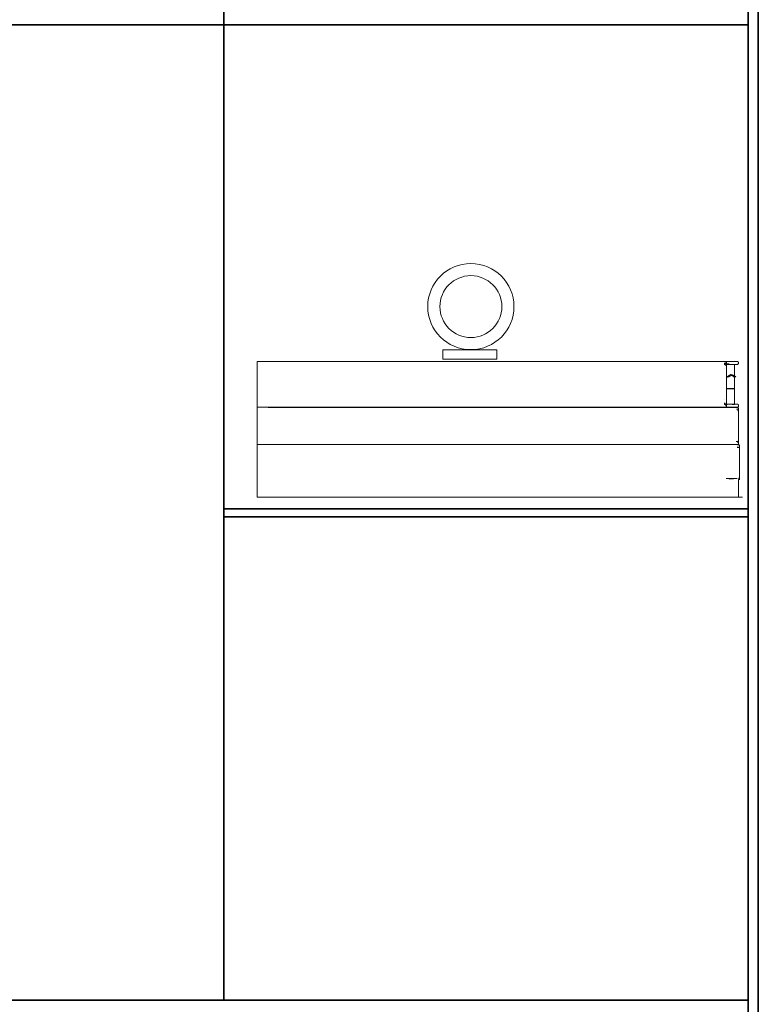
# Model space of a CAD drawing. Units: millimetres. Extents: x 2322 to 2394, y 1600 to 1790.
# Tile 3 of 5: x 2358 to 2394, y 1648 to 1696. Entities that reach past the tile are written whole.
import ezdxf

# ---------------------------------------------------------------- set-up
doc = ezdxf.new("R2010")
doc.units = ezdxf.units.MM
doc.layers.add('A-FURN', color=7, linetype='Continuous', lineweight=35)
doc.layers.add('A-FURN-ACCS', color=8, linetype='Continuous', lineweight=18)

msp = doc.modelspace()

# ---------------------------------------------------------------- linework, layer by layer
at = {"layer": 'A-FURN'}
for p, q in [((2393.58, 1755.925), (2393.58, 1599.925)), ((2393.08, 1755.425), (2393.08, 1600.425)), ((2367.535, 1701.437), (2367.535, 1648.381)), ((2322.08, 1695.937), (2393.08, 1695.937)), ((2393.08, 1695.937), (2393.08, 1600.425)), ((2393.08, 1695.937), (2393.08, 1648.381)), ((2367.535, 1672.346), (2393.08, 1672.346)), ((2367.535, 1671.946), (2393.08, 1671.946)), ((2393.08, 1648.381), (2322.08, 1648.381))]:
    msp.add_line(p, q, dxfattribs=at)
at = {"layer": 'A-FURN-ACCS'}
for p, q in [((2391.983, 1679.528), (2369.151, 1679.528)), ((2369.151, 1679.528), (2369.151, 1672.902)), ((2391.992, 1679.442), (2391.91, 1679.442)), ((2391.915, 1679.412), (2391.91, 1679.413)), ((2391.91, 1679.377), (2391.978, 1679.377)), ((2391.922, 1679.33), (2391.91, 1679.33)), ((2392.007, 1679.413), (2391.915, 1679.412)), ((2391.985, 1679.37), (2391.978, 1679.37)), ((2391.992, 1679.33), (2391.978, 1679.33)), ((2392.002, 1679.512), (2391.983, 1679.528)), ((2392.567, 1679.528), (2391.983, 1679.528)), ((2391.988, 1679.373), (2391.985, 1679.37)), ((2392.014, 1679.422), (2391.992, 1679.442)), ((2392.028, 1679.363), (2391.992, 1679.33)), ((2392.002, 1679.512), (2392.027, 1679.494)), ((2392.029, 1679.408), (2392.025, 1679.412)), ((2392.025, 1679.412), (2392.029, 1679.412)), ((2392.029, 1679.405), (2392.025, 1679.401)), ((2392.025, 1679.377), (2392.029, 1679.405)), ((2392.028, 1679.372), (2392.025, 1679.377)), ((2392.028, 1679.377), (2392.025, 1679.377)), ((2392.027, 1679.49), (2392.027, 1679.494)), ((2392.03, 1679.488), (2392.027, 1679.49)), ((2392.027, 1679.109), (2392.028, 1679.324)), ((2392.039, 1679.374), (2392.028, 1679.377)), ((2392.028, 1679.363), (2392.028, 1679.372)), ((2392.037, 1679.372), (2392.028, 1679.363)), ((2392.028, 1679.324), (2392.028, 1679.363)), ((2392.029, 1679.412), (2392.032, 1679.454)), ((2392.029, 1679.412), (2392.036, 1679.414)), ((2392.029, 1679.408), (2392.029, 1679.412)), ((2392.037, 1679.4), (2392.029, 1679.408)), ((2392.029, 1679.405), (2392.029, 1679.408)), ((2392.032, 1679.454), (2392.03, 1679.488)), ((2392.036, 1679.414), (2392.032, 1679.454)), ((2392.045, 1679.419), (2392.036, 1679.414)), ((2392.036, 1679.414), (2392.044, 1679.413)), ((2392.037, 1679.4), (2392.036, 1679.414)), ((2392.037, 1679.372), (2392.039, 1679.374)), ((2392.039, 1679.374), (2392.04, 1679.385)), ((2392.039, 1679.374), (2392.055, 1679.377)), ((2392.04, 1679.385), (2392.043, 1679.408)), ((2392.043, 1679.408), (2392.044, 1679.413)), ((2392.044, 1679.413), (2392.045, 1679.419)), ((2392.044, 1679.413), (2392.053, 1679.413)), ((2392.055, 1679.377), (2392.421, 1679.377)), ((2392.078, 1679.412), (2392.068, 1679.413)), ((2392.163, 1679.413), (2392.078, 1679.412)), ((2392.421, 1679.377), (2392.419, 1679.179)), ((2392.421, 1679.377), (2392.567, 1679.377)), ((2392.567, 1679.528), (2392.612, 1679.486)), ((2392.612, 1679.419), (2392.567, 1679.377)), ((2392.612, 1679.486), (2392.612, 1679.419)), ((2391.913, 1679.179), (2391.909, 1679.179)), ((2392.025, 1678.791), (2392.027, 1679.109)), ((2392.027, 1678.788), (2392.025, 1678.791)), ((2392.025, 1678.788), (2392.025, 1678.791)), ((2392.025, 1678.788), (2392.027, 1678.788)), ((2392.025, 1678.779), (2392.025, 1678.788)), ((2392.025, 1678.779), (2392.027, 1678.779)), ((2392.025, 1678.775), (2392.025, 1678.779)), ((2392.025, 1678.775), (2392.093, 1678.776)), ((2392.025, 1678.768), (2392.025, 1678.775)), ((2392.071, 1678.791), (2392.027, 1678.788)), ((2392.027, 1678.779), (2392.093, 1678.776)), ((2392.071, 1678.791), (2392.074, 1678.788)), ((2392.074, 1678.788), (2392.079, 1678.791)), ((2392.083, 1678.791), (2392.079, 1678.791)), ((2392.166, 1678.777), (2392.079, 1678.768)), ((2392.093, 1678.776), (2392.079, 1678.768)), ((2392.083, 1678.791), (2392.237, 1678.882)), ((2392.093, 1678.776), (2392.096, 1678.779)), ((2392.166, 1678.777), (2392.096, 1678.779)), ((2392.237, 1678.859), (2392.164, 1678.817)), ((2392.166, 1678.777), (2392.275, 1678.84)), ((2392.329, 1678.87), (2392.237, 1678.882)), ((2392.237, 1678.882), (2392.273, 1678.863)), ((2392.273, 1678.863), (2392.237, 1678.859)), ((2392.259, 1678.848), (2392.237, 1678.859)), ((2392.329, 1678.87), (2392.273, 1678.863)), ((2392.273, 1678.863), (2392.286, 1678.857)), ((2392.275, 1678.84), (2392.296, 1678.852)), ((2392.372, 1678.791), (2392.275, 1678.84)), ((2392.296, 1678.852), (2392.329, 1678.87)), ((2392.296, 1678.852), (2392.382, 1678.808)), ((2392.417, 1678.82), (2392.329, 1678.87)), ((2392.397, 1678.791), (2392.372, 1678.791)), ((2392.395, 1678.779), (2392.372, 1678.791)), ((2392.395, 1678.779), (2392.407, 1678.779)), ((2392.417, 1678.768), (2392.395, 1678.779)), ((2392.419, 1679.179), (2392.417, 1678.921)), ((2392.417, 1678.921), (2392.417, 1678.82)), ((2392.49, 1678.779), (2392.417, 1678.82)), ((2392.49, 1678.779), (2392.417, 1678.768)), ((2392.024, 1678.21), (2392.027, 1678.652)), ((2392.025, 1678.768), (2392.027, 1678.765)), ((2392.025, 1678.765), (2392.025, 1678.768)), ((2392.027, 1678.765), (2392.025, 1678.765)), ((2392.027, 1678.652), (2392.025, 1678.765)), ((2392.074, 1678.765), (2392.027, 1678.765)), ((2392.079, 1678.768), (2392.074, 1678.765)), ((2392.417, 1678.768), (2392.416, 1678.638)), ((2392.416, 1678.21), (2392.416, 1678.638)), ((2392.024, 1678.187), (2392.024, 1678.21)), ((2392.024, 1678.21), (2392.074, 1678.21)), ((2392.027, 1678.142), (2392.024, 1678.187)), ((2392.027, 1678.187), (2392.024, 1678.187)), ((2392.027, 1678.187), (2392.074, 1678.187)), ((2392.027, 1678.142), (2392.028, 1677.498)), ((2392.074, 1678.21), (2392.416, 1678.21)), ((2392.074, 1678.187), (2392.417, 1678.187)), ((2392.416, 1678.21), (2392.271, 1678.198)), ((2392.271, 1678.198), (2392.417, 1678.187)), ((2392.417, 1677.914), (2392.417, 1678.187)), ((2392.417, 1677.914), (2392.419, 1677.657)), ((2391.909, 1677.657), (2391.913, 1677.657)), ((2391.966, 1677.492), (2391.91, 1677.492)), ((2391.979, 1677.451), (2391.91, 1677.451)), ((2391.91, 1677.445), (2391.993, 1677.445)), ((2391.926, 1677.424), (2392.006, 1677.422)), ((2392.006, 1677.422), (2391.928, 1677.422)), ((2391.986, 1677.379), (2391.962, 1677.379)), ((2391.993, 1677.445), (2391.988, 1677.449)), ((2391.999, 1677.445), (2391.993, 1677.445)), ((2391.999, 1677.445), (2392.011, 1677.434)), ((2392.01, 1677.432), (2391.999, 1677.445)), ((2392.017, 1677.445), (2391.999, 1677.445)), ((2392.028, 1677.458), (2392.023, 1677.462)), ((2392.025, 1677.445), (2392.028, 1677.45)), ((2392.028, 1677.445), (2392.025, 1677.445)), ((2392.025, 1677.424), (2392.025, 1677.445)), ((2392.025, 1677.424), (2392.029, 1677.422)), ((2392.029, 1677.422), (2392.025, 1677.422)), ((2392.029, 1677.414), (2392.025, 1677.41)), ((2392.028, 1677.458), (2392.028, 1677.498)), ((2392.028, 1677.45), (2392.028, 1677.458)), ((2392.037, 1677.45), (2392.028, 1677.458)), ((2392.039, 1677.448), (2392.028, 1677.445)), ((2392.029, 1677.417), (2392.029, 1677.422)), ((2392.037, 1677.422), (2392.029, 1677.417)), ((2392.037, 1677.422), (2392.029, 1677.422)), ((2392.029, 1677.417), (2392.029, 1677.414)), ((2392.029, 1677.414), (2392.032, 1677.365)), ((2392.029, 1677.414), (2392.036, 1677.409)), ((2392.03, 1677.333), (2392.032, 1677.365)), ((2392.032, 1677.365), (2392.036, 1677.409)), ((2392.036, 1677.409), (2392.037, 1677.422)), ((2392.036, 1677.409), (2392.045, 1677.403)), ((2392.039, 1677.448), (2392.037, 1677.45)), ((2392.055, 1677.445), (2392.039, 1677.448)), ((2392.04, 1677.436), (2392.039, 1677.448)), ((2392.043, 1677.414), (2392.04, 1677.436)), ((2392.045, 1677.403), (2392.043, 1677.414)), ((2392.424, 1677.445), (2392.055, 1677.445)), ((2392.305, 1677.423), (2392.308, 1677.422)), ((2392.421, 1677.422), (2392.308, 1677.422)), ((2392.419, 1677.657), (2392.424, 1677.445)), ((2392.424, 1677.445), (2392.421, 1677.422)), ((2392.424, 1677.445), (2392.567, 1677.445)), ((2392.567, 1677.445), (2392.612, 1677.403)), ((2392.612, 1677.336), (2392.567, 1677.294)), ((2392.612, 1677.403), (2392.612, 1677.336)), ((2391.983, 1677.294), (2369.151, 1677.294)), ((2392.576, 1677.287), (2369.688, 1677.287)), ((2391.983, 1677.294), (2392.027, 1677.328)), ((2391.983, 1677.294), (2392.567, 1677.294)), ((2392.027, 1677.328), (2392.03, 1677.333)), ((2392.576, 1677.203), (2392.523, 1677.203)), ((2392.576, 1677.287), (2392.622, 1677.246)), ((2392.622, 1677.248), (2392.576, 1677.287)), ((2392.576, 1677.287), (2392.622, 1677.253)), ((2392.61, 1677.172), (2392.576, 1677.203)), ((2392.61, 1677.172), (2392.576, 1677.14)), ((2392.619, 1677.164), (2392.576, 1677.133)), ((2392.622, 1677.135), (2392.576, 1677.094)), ((2392.622, 1677.183), (2392.61, 1677.172)), ((2392.619, 1677.164), (2392.61, 1677.172)), ((2392.619, 1677.164), (2392.622, 1677.17)), ((2392.622, 1677.166), (2392.619, 1677.164)), ((2392.622, 1677.162), (2392.619, 1677.164)), ((2392.622, 1677.248), (2392.622, 1677.253)), ((2392.622, 1677.246), (2392.622, 1677.248)), ((2392.622, 1677.183), (2392.622, 1677.246)), ((2392.622, 1677.17), (2392.622, 1677.183)), ((2392.622, 1677.17), (2392.622, 1677.166)), ((2392.622, 1677.166), (2392.622, 1677.162)), ((2392.622, 1677.164), (2392.622, 1677.166)), ((2392.622, 1677.162), (2392.622, 1677.164)), ((2392.622, 1677.135), (2392.622, 1677.162)), ((2392.622, 1677.135), (2392.622, 1675.515)), ((2392.576, 1675.482), (2369.151, 1675.482)), ((2369.151, 1675.473), (2392.597, 1675.473)), ((2392.508, 1675.629), (2392.576, 1675.629)), ((2392.576, 1675.566), (2392.56, 1675.566)), ((2392.583, 1675.668), (2392.576, 1675.675)), ((2392.576, 1675.629), (2392.603, 1675.605)), ((2392.59, 1675.579), (2392.576, 1675.566)), ((2392.622, 1675.515), (2392.576, 1675.482)), ((2392.606, 1675.613), (2392.581, 1675.631)), ((2392.597, 1675.473), (2392.617, 1675.455)), ((2392.616, 1675.473), (2392.597, 1675.473)), ((2392.617, 1675.637), (2392.611, 1675.643)), ((2392.616, 1675.473), (2392.661, 1675.44)), ((2392.644, 1675.427), (2392.646, 1675.414)), ((2392.646, 1675.414), (2392.647, 1675.393)), ((2392.66, 1675.386), (2392.661, 1675.44)), ((2392.661, 1675.44), (2392.663, 1675.384)), ((2392.566, 1675.39), (2392.551, 1675.39)), ((2392.597, 1675.326), (2392.551, 1675.326)), ((2392.624, 1675.324), (2392.62, 1675.326)), ((2392.624, 1675.324), (2392.651, 1675.349)), ((2392.649, 1675.351), (2392.642, 1675.356)), ((2392.651, 1675.322), (2392.645, 1675.316)), ((2392.649, 1675.364), (2392.649, 1675.351)), ((2392.649, 1675.351), (2392.651, 1675.349)), ((2392.651, 1675.349), (2392.656, 1675.348)), ((2392.652, 1675.329), (2392.651, 1675.322)), ((2392.656, 1675.348), (2392.652, 1675.329)), ((2392.657, 1675.353), (2392.656, 1675.348)), ((2392.657, 1675.353), (2392.66, 1675.378)), ((2392.663, 1675.384), (2392.664, 1675.101)), ((2392.664, 1675.101), (2392.665, 1674.76)), ((2392.665, 1674.76), (2392.665, 1674.368)), ((2392.665, 1674.368), (2392.664, 1673.833)), ((2392.373, 1673.816), (2392.015, 1673.816)), ((2392.372, 1673.794), (2392.161, 1673.793)), ((2392.373, 1673.816), (2392.372, 1673.794)), ((2392.552, 1673.816), (2392.373, 1673.816)), ((2392.651, 1673.793), (2392.619, 1673.817)), ((2392.649, 1673.79), (2392.619, 1673.765)), ((2392.619, 1673.765), (2392.619, 1672.902)), ((2392.651, 1673.82), (2392.625, 1673.843)), ((2392.648, 1673.77), (2392.647, 1673.749)), ((2392.649, 1673.79), (2392.648, 1673.77)), ((2392.651, 1673.793), (2392.649, 1673.79)), ((2392.651, 1673.82), (2392.652, 1673.813)), ((2392.657, 1673.792), (2392.651, 1673.793)), ((2392.652, 1673.813), (2392.655, 1673.797)), ((2392.655, 1673.797), (2392.657, 1673.792)), ((2392.657, 1673.792), (2392.659, 1673.789)), ((2392.659, 1673.789), (2392.66, 1673.756)), ((2392.663, 1673.758), (2392.66, 1673.756)), ((2392.664, 1673.833), (2392.663, 1673.758)), ((2369.151, 1672.902), (2392.818, 1672.902))]:
    msp.add_line(p, q, dxfattribs=at)
msp.add_lwpolyline([(2378.21, 1680.096), (2380.83, 1680.096), (2380.83, 1679.628), (2378.21, 1679.628)], close=True, dxfattribs=at)
for radius in [2.101, 1.509]:
    msp.add_circle((2379.571, 1682.2), radius, dxfattribs=at)

doc.saveas('drawing.dxf')
